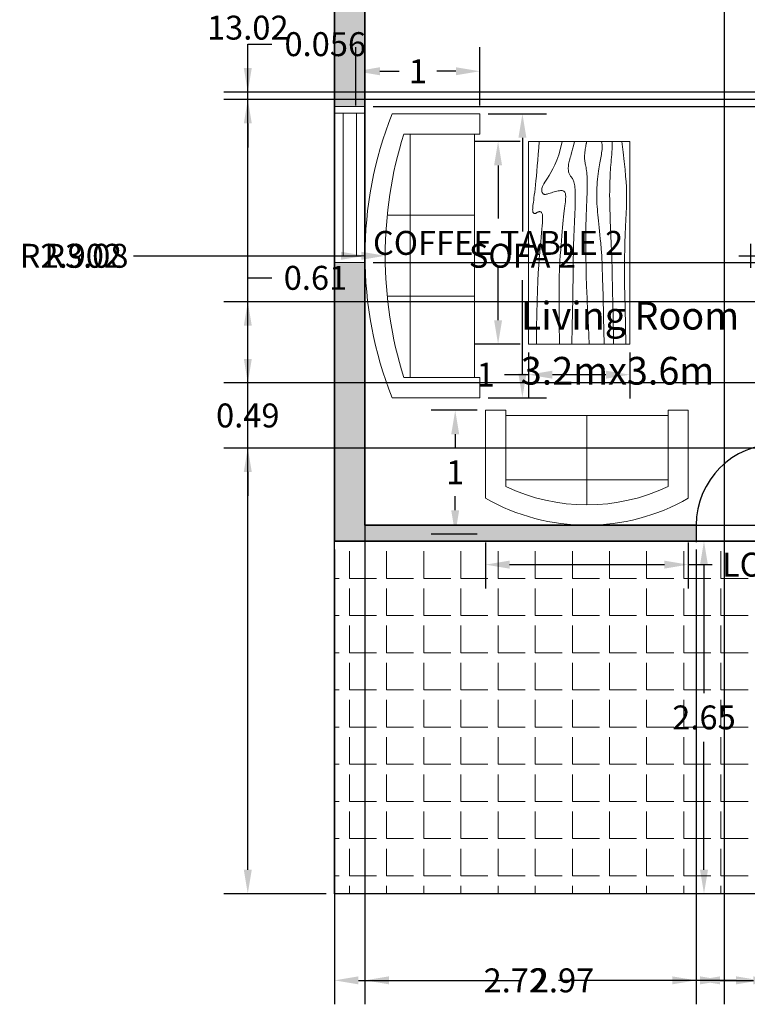
# Model space of a CAD drawing. Units: metres. Extents: x 35.2 to 46.4, y 446.1 to 460.8.
# Tile 1 of 6: x 35.2 to 40.7, y 446.1 to 453.5. Entities that reach past the tile are written whole.
import ezdxf

# ---------------------------------------------------------------- set-up
doc = ezdxf.new("R2010")
doc.units = ezdxf.units.M
for name, color, linetype, lineweight in [('A-ANNO-DIMS', 2, 'Continuous', 18), ('A-AREA-IDEN', 7, 'Continuous', 18), ('A-DOOR', 3, 'Continuous', 25), ('A-FLOR', 7, 'Continuous', 25), ('A-FLOR-PATT', 9, 'Continuous', 13), ('A-GLAZ', 4, 'Continuous', 18), ('A-WALL', 7, 'Continuous', 35), ('A-WALL-PATT', 252, 'Continuous', 13), ('FURNITURE', 53, 'Continuous', 18)]:
    doc.layers.add(name, color=color, linetype=linetype, lineweight=lineweight)
doc.styles.get("Standard").update_dxf_attribs({"font": 'calibri.ttf'})
doc.dimstyles.get("Standard").update_dxf_attribs({"dimtxt": 0.18, "dimasz": 0.18, "dimexe": 0.18, "dimexo": 0.0625, "dimgap": 0.09, "dimtad": 0, "dimtih": 1, "dimtoh": 1, "dimdec": 4, "dimzin": 0, "dimdsep": 46, "dimtxsty": 'Standard', "dimcen": 0.09, "dimadec": 0, "dimazin": 0, "dimtfac": 1, "dimtdec": 4, "dimtofl": 0, "dimtmove": 0, "dimatfit": 3, "dimfxl": 1, "dimtolj": 1, "dimtzin": 0, "dimarcsym": 0})

# ---------------------------------------------------------------- blocks, each defined once
blk = doc.blocks.new('*U4')
for p, q in [((-24, 0), (-24, -5)), ((0, 0), (0, -5))]:
    blk.add_line(p, q)
blk.add_lwpolyline([(0, 0), (0, 24), (-1.75, 24), (-1.75, 0)], close=True)
blk.add_arc((0, 0), 24, 90, 180)
blk = doc.blocks.new('Table - Rectangular Woodgrain 60 x 30 in.')
for p, q in [((0, 0), (0, -30)), ((60, 0), (0, 0)), ((60, -30), (60, 0)), ((0, -30), (60, -30))]:
    blk.add_line(p, q)
for points in [[(0, -2.4), (4.8155, -2.418), (9.0302, -2.4688), (12.709, -2.5477), (15.9167, -2.65), (18.7181, -2.7711), (21.1781, -2.9063), (23.3616, -3.0508), (25.3333, -3.2), (27.1477, -3.3495), (28.8172, -3.4958), (30.3437, -3.636), (31.7291, -3.7667), (32.9756, -3.8849), (34.0849, -3.9875), (35.059, -4.0714), (35.9, -4.1334), (36.6114, -4.1711), (37.2041, -4.1854), (37.6906, -4.1779), (38.0833, -4.15), (38.3948, -4.1034), (38.6375, -4.0396), (38.8239, -3.9602), (38.9666, -3.8667), (39.0764, -3.7608), (39.1573, -3.6448), (39.2116, -3.521), (39.2416, -3.3917), (39.2498, -3.2593), (39.2385, -3.1261), (39.21, -2.9944), (39.1666, -2.8667), (39.111, -2.7447), (39.0468, -2.6281), (38.978, -2.5163), (38.9083, -2.4083), (38.8418, -2.3035), (38.7823, -2.201), (38.7337, -2.1001), (38.7, -2), (38.6844, -1.9003), (38.6875, -1.8021), (38.7094, -1.707), (38.75, -1.6167), (38.8094, -1.5326), (38.8875, -1.4563), (38.9844, -1.3893), (39.1, -1.3333), (39.2351, -1.2896), (39.3937, -1.2583), (39.5804, -1.2396), (39.8, -1.2333), (40.057, -1.2396), (40.3562, -1.2583), (40.7023, -1.2896), (41.1, -1.3333), (41.5547, -1.3895), (42.0755, -1.4573), (42.6721, -1.5361), (43.3542, -1.625), (44.1316, -1.7233), (45.014, -1.8302), (46.0114, -1.9449), (47.1333, -2.0667), (48.3862, -2.1947), (49.7625, -2.3281), (51.2513, -2.4663), (52.8416, -2.6083), (54.5226, -2.7535), (56.2833, -2.9011), (58.1127, -3.0501), (60, -3.2)], [(0, -9.2), (6.5759, -9.0858), (11.9385, -9.0365), (16.2527, -9.0418), (19.6833, -9.0917), (22.3952, -9.1759), (24.5531, -9.2844), (26.322, -9.4069), (27.8666, -9.5333), (29.3241, -9.6553), (30.7203, -9.7719), (32.0532, -9.8837), (33.3208, -9.9917), (34.5213, -10.0965), (35.6526, -10.199), (36.7128, -10.2999), (37.7, -10.4), (38.6129, -10.4996), (39.4531, -10.5969), (40.223, -10.6895), (40.925, -10.775), (41.5613, -10.8512), (42.1344, -10.9156), (42.6465, -10.966), (43.1, -11), (43.4976, -11.0158), (43.8437, -11.0136), (44.143, -10.9942), (44.4, -10.9583), (44.6195, -10.9069), (44.8062, -10.8406), (44.9648, -10.7603), (45.1, -10.6667), (45.2155, -10.5598), (45.3114, -10.4365), (45.3871, -10.2929), (45.4416, -10.125), (45.4743, -9.929), (45.4844, -9.7011), (45.4709, -9.4371), (45.4333, -9.1333), (45.3716, -8.7883), (45.2896, -8.4104), (45.1919, -8.0107), (45.0833, -7.6), (44.9685, -7.1893), (44.8521, -6.7896), (44.7388, -6.4117), (44.6333, -6.0667), (44.54, -5.7628), (44.4614, -5.4979), (44.4001, -5.2675), (44.3583, -5.0667), (44.3384, -4.8909), (44.3427, -4.7354), (44.3736, -4.5956), (44.4333, -4.4667), (44.5236, -4.3453), (44.6427, -4.2333), (44.7884, -4.1339), (44.9583, -4.05), (45.1501, -3.9849), (45.3614, -3.9417), (45.59, -3.9234), (45.8333, -3.9333), (46.0915, -3.9749), (46.3734, -4.0531), (46.6906, -4.1736), (47.0542, -4.3417), (47.4756, -4.5629), (47.9661, -4.8427), (48.5372, -5.1866), (49.2, -5.6), (49.9676, -6.0844), (50.8594, -6.625), (51.8965, -7.2031), (53.1, -7.8), (54.491, -8.3969), (56.0906, -8.975), (57.9199, -9.5156), (60, -10)], [(0, -12.8), (5.1847, -12.9322), (9.6213, -13.0323), (13.3963, -13.1059), (16.5958, -13.1583), (19.3063, -13.1952), (21.614, -13.2219), (23.6054, -13.2439), (25.3666, -13.2667), (26.9728, -13.2947), (28.4531, -13.3281), (29.8256, -13.3663), (31.1083, -13.4083), (32.3191, -13.4535), (33.476, -13.501), (34.597, -13.5501), (35.7, -13.6), (36.7984, -13.6497), (37.8875, -13.6979), (38.9578, -13.743), (40, -13.7833), (41.0047, -13.8174), (41.9625, -13.8438), (42.864, -13.8607), (43.7, -13.8667), (44.4631, -13.8604), (45.1552, -13.8417), (45.7801, -13.8104), (46.3416, -13.7667), (46.8439, -13.7104), (47.2906, -13.6417), (47.6858, -13.5604), (48.0333, -13.4667), (48.3375, -13.3608), (48.6042, -13.2448), (48.8396, -13.121), (49.05, -12.9917), (49.2417, -12.8593), (49.4208, -12.7261), (49.5937, -12.5944), (49.7667, -12.4667), (49.9452, -12.3451), (50.1323, -12.2313), (50.3303, -12.1268), (50.5416, -12.0333), (50.7686, -11.9524), (51.0135, -11.8854), (51.2788, -11.8341), (51.5666, -11.8), (51.8785, -11.7843), (52.2116, -11.7865), (52.562, -11.8059), (52.926, -11.8417), (53.2998, -11.8931), (53.6795, -11.9594), (54.0614, -12.0397), (54.4416, -12.1333), (54.8223, -12.2401), (55.2293, -12.3625), (55.6942, -12.5037), (56.2489, -12.6667), (56.9251, -12.8547), (57.7545, -13.0708), (58.7689, -13.3182), (60, -13.6)], [(0, -18), (5.124, -17.7273), (9.6609, -17.5057), (13.6705, -17.3303), (17.2125, -17.1958), (20.3467, -17.0973), (23.1328, -17.0297), (25.6307, -16.9878), (27.9, -16.9667), (29.9928, -16.9617), (31.9302, -16.9703), (33.7254, -16.9907), (35.3917, -17.0208), (36.9423, -17.0588), (38.3906, -17.1026), (39.7499, -17.1503), (41.0333, -17.2), (42.2519, -17.2496), (43.4073, -17.2969), (44.4986, -17.3395), (45.525, -17.375), (46.4858, -17.4012), (47.3802, -17.4156), (48.2074, -17.416), (48.9667, -17.4), (49.6583, -17.3662), (50.2872, -17.3167), (50.8595, -17.2547), (51.3812, -17.1833), (51.8584, -17.1057), (52.2971, -17.025), (52.7034, -16.9443), (53.0833, -16.8667), (53.443, -16.7951), (53.789, -16.7313), (54.128, -16.6768), (54.4666, -16.6334), (54.8115, -16.6024), (55.1693, -16.5854), (55.5465, -16.5841), (55.95, -16.6), (56.3828, -16.6337), (56.8346, -16.6823), (57.2915, -16.7418), (57.7396, -16.8084), (58.165, -16.878), (58.5539, -16.9469), (58.8924, -17.0111), (59.1666, -17.0667), (59.3679, -17.1107), (59.5078, -17.1438), (59.6032, -17.1675), (59.6708, -17.1833), (59.7275, -17.193), (59.7901, -17.1979), (59.8753, -17.1998), (60, -17.2)], [(0, -22.4), (8.0098, -22.2501), (14.4094, -22.1011), (19.4168, -21.9535), (23.25, -21.8083), (26.1269, -21.6663), (28.2656, -21.5281), (29.884, -21.3947), (31.2, -21.2667), (32.3967, -21.1448), (33.5172, -21.0292), (34.5697, -20.9198), (35.5625, -20.8167), (36.5037, -20.7198), (37.4015, -20.6292), (38.2642, -20.5448), (39.1, -20.4667), (39.9164, -20.3951), (40.7187, -20.3313), (41.5117, -20.2768), (42.3, -20.2333), (43.0883, -20.2024), (43.8812, -20.1854), (44.6836, -20.1841), (45.5, -20.2), (46.3328, -20.234), (47.1747, -20.2844), (48.0163, -20.3488), (48.8479, -20.425), (49.66, -20.5106), (50.4429, -20.6031), (51.1872, -20.7004), (51.8833, -20.8), (52.5246, -20.8999), (53.1166, -20.9995), (53.6681, -21.0983), (54.1875, -21.1958), (54.6834, -21.2919), (55.1646, -21.3859), (55.6394, -21.4777), (56.1167, -21.5667), (56.6028, -21.6515), (57.0961, -21.7266), (57.5929, -21.7852), (58.0896, -21.8208), (58.5823, -21.8268), (59.0674, -21.7964), (59.5412, -21.723), (60, -21.6)], [(0, -25.2), (8.6355, -25.0504), (15.7026, -24.9031), (21.4049, -24.7606), (25.9458, -24.625), (29.529, -24.4988), (32.3578, -24.3844), (34.6359, -24.284), (36.5667, -24.2), (38.3213, -24.1341), (39.9417, -24.0854), (41.437, -24.0523), (42.8167, -24.0333), (44.0901, -24.0268), (45.2667, -24.0313), (46.3557, -24.0451), (47.3667, -24.0667), (48.309, -24.0947), (49.1928, -24.1287), (50.0284, -24.168), (50.826, -24.2125), (51.5959, -24.2617), (52.3483, -24.3151), (53.0935, -24.3725), (53.8417, -24.4334), (54.6009, -24.497), (55.3699, -24.561), (56.1454, -24.6226), (56.9239, -24.6792), (57.7021, -24.7279), (58.4764, -24.7662), (59.2435, -24.7911), (60, -24.8)], [(0, -28.8), (5.6867, -28.6681), (10.45, -28.5698), (14.407, -28.5012), (17.675, -28.4584), (20.3711, -28.4374), (22.6125, -28.4344), (24.5164, -28.4455), (26.2, -28.4667), (27.762, -28.4947), (29.2276, -28.5281), (30.6033, -28.5663), (31.8958, -28.6084), (33.1118, -28.6535), (34.2578, -28.7011), (35.3405, -28.7501), (36.3666, -28.8), (37.3443, -28.8497), (38.288, -28.8974), (39.2137, -28.9412), (40.1375, -28.9792), (41.0753, -29.0093), (42.0432, -29.0297), (43.0572, -29.0384), (44.1333, -29.0333), (45.2936, -29.0114), (46.5843, -28.9641), (48.0579, -28.8816), (49.7666, -28.7542), (51.7629, -28.5721), (54.0989, -28.3255), (56.8272, -28.0048), (60, -27.6)]]:
    blk.add_lwpolyline(points)
blk = doc.blocks.new('Sofa - Roundback 7 ft.')
for p, q in [((-12.00002, -32.4421), (-12.00003, -6.5971)), ((11.99997, -32.4421), (11.99998, -6.5971)), ((-36.000027, -34), (-36.000027, -11.4696)), ((35.99998, -34), (35.99998, -11.4696)), ((-35.999844, -13.3819), (35.9998, -13.3819)), ((-36.000027, -32.4421), (35.99998, -32.4421))]:
    blk.add_line(p, q)
for points in [[(-36.000027, -34), (-42.000027, -34), (-42.000027, -8)], [(41.99998, -8), (41.99998, -34), (35.99998, -34)]]:
    blk.add_lwpolyline(points)
for centre, radius, start, end in [((0, -114.25), 114.25, 68.43141, 111.5686), ((-0.00001, -127.1968), 121.1968, 72.72033, 107.2797)]:
    blk.add_arc(centre, radius, start, end)
blk = doc.blocks.new('Sofa - Roundback Loveseat 5 ft.')
for p, q in [((0, -32.44198), (0, -5.99998)), ((-24, -33.99998), (-24, -11.46958)), ((24.00004, -33.99998), (24.00004, -11.46958)), ((-23.9998, -13.38178), (23.99986, -13.38178)), ((-24, -32.44198), (24.00004, -32.44198))]:
    blk.add_line(p, q)
for points in [[(-24, -33.99998), (-30, -33.99998), (-30, -7.99998)], [(30.00004, -7.99998), (30.00004, -33.99998), (24.00004, -33.99998)]]:
    blk.add_lwpolyline(points)
for centre, radius, start, end in [((0, -60.24998), 60.24998, 60.13715, 119.8628), ((0, -61.38438), 55.38444, 64.32083, 115.6792)]:
    blk.add_arc(centre, radius, start, end)
blk = doc.blocks.new('WIN-1172')
for p, q in [((0, 1.1716), (0.23, 1.1716)), ((0, 1.1716), (0, 0)), ((0, 1.1216), (0.23, 1.1216)), ((0.065, 1.1216), (0.065, 0.05)), ((0.165, 1.1216), (0.165, 0.05)), ((0.23, 1.1716), (0.23, 0)), ((0.23, 0.05), (0, 0.05)), ((0.23, 0), (0, 0))]:
    blk.add_line(p, q)
blk = doc.blocks.new('*D141')
at = {"layer": 'A-ANNO-DIMS', "color": 0, "lineweight": -2, "transparency": 16777216}
for p, q in [((39.0034, 452.5589), (38.6573, 452.5589)), ((38.8373, 452.3789), (38.8373, 451.9792)), ((38.8373, 451.2149), (38.8373, 451.6147)), ((39.0034, 451.0349), (38.6573, 451.0349))]:
    blk.add_line(p, q, dxfattribs=at)
at = {"layer": 'A-ANNO-DIMS', "color": 0, "transparency": 16777216}
for points in [[(38.8073, 452.3789), (38.8673, 452.3789), (38.8373, 452.5589)], [(38.8073, 451.2149), (38.8673, 451.2149), (38.8373, 451.0349)]]:
    blk.add_solid(points, dxfattribs=at)
at = {"layer": 'Defpoints', "color": 0, "transparency": 16777216}
for p in [(38.8373, 452.5589), (39.0659, 452.5589), (39.0659, 451.0349)]:
    blk.add_point(p, dxfattribs=at)
at = {"layer": 'A-ANNO-DIMS', "color": 0, "transparency": 16777216, "insert": (38.8373, 451.7969), "char_height": 0.18, "attachment_point": 5}
blk.add_mtext('\\A1;COFFEE TABLE 2', dxfattribs=at)
blk = doc.blocks.new('*D142')
at = {"layer": 'A-ANNO-DIMS', "color": 0, "lineweight": -2, "transparency": 16777216}
for p, q in [((39.0659, 450.9724), (39.0659, 450.6263)), ((39.8279, 450.9724), (39.8279, 450.6263)), ((39.0659, 450.8063), (38.8859, 450.8063)), ((39.6479, 450.8063), (39.2459, 450.8063))]:
    blk.add_line(p, q, dxfattribs=at)
at = {"layer": 'A-ANNO-DIMS', "color": 0, "transparency": 16777216}
for points in [[(39.2459, 450.8363), (39.2459, 450.7763), (39.0659, 450.8063)], [(39.6479, 450.8363), (39.6479, 450.7763), (39.8279, 450.8063)]]:
    blk.add_solid(points, dxfattribs=at)
at = {"layer": 'Defpoints', "color": 0, "transparency": 16777216}
for p in [(39.0659, 451.0349), (39.8279, 451.0349), (39.0659, 450.8063)]:
    blk.add_point(p, dxfattribs=at)
at = {"layer": 'A-ANNO-DIMS', "color": 0, "transparency": 16777216, "insert": (38.7437, 450.8063), "char_height": 0.18, "attachment_point": 5}
blk.add_mtext('\\A1;1', dxfattribs=at)
blk = doc.blocks.new('*D143')
at = {"layer": 'A-ANNO-DIMS', "color": 0, "lineweight": -2, "transparency": 16777216}
for p, q in [((38.7627, 452.7669), (39.2002, 452.7669)), ((39.0202, 452.5869), (39.0202, 451.8824)), ((39.0202, 450.8133), (39.0202, 451.5179)), ((38.7627, 450.6333), (39.2002, 450.6333))]:
    blk.add_line(p, q, dxfattribs=at)
at = {"layer": 'A-ANNO-DIMS', "color": 0, "transparency": 16777216}
for points in [[(38.9902, 452.5869), (39.0502, 452.5869), (39.0202, 452.7669)], [(38.9902, 450.8133), (39.0502, 450.8133), (39.0202, 450.6333)]]:
    blk.add_solid(points, dxfattribs=at)
at = {"layer": 'Defpoints', "color": 0, "transparency": 16777216}
for p in [(38.7002, 452.7669), (39.0202, 452.7669), (38.7002, 450.6333)]:
    blk.add_point(p, dxfattribs=at)
at = {"layer": 'A-ANNO-DIMS', "color": 0, "transparency": 16777216, "insert": (39.0202, 451.7001), "char_height": 0.18, "attachment_point": 5}
blk.add_mtext('\\A1;SOFA 2', dxfattribs=at)
blk = doc.blocks.new('*D144')
at = {"layer": 'A-ANNO-DIMS', "color": 0, "lineweight": -2, "transparency": 16777216}
for p, q in [((37.7689, 452.8294), (37.7689, 453.267)), ((38.7002, 452.8294), (38.7002, 453.267)), ((37.9489, 453.087), (38.0924, 453.087)), ((38.5202, 453.087), (38.3767, 453.087))]:
    blk.add_line(p, q, dxfattribs=at)
at = {"layer": 'A-ANNO-DIMS', "color": 0, "transparency": 16777216}
for points in [[(37.9489, 453.117), (37.9489, 453.057), (37.7689, 453.087)], [(38.5202, 453.117), (38.5202, 453.057), (38.7002, 453.087)]]:
    blk.add_solid(points, dxfattribs=at)
at = {"layer": 'Defpoints', "color": 0, "transparency": 16777216}
for p in [(37.7689, 453.087), (37.7689, 452.7669), (38.7002, 452.7669)]:
    blk.add_point(p, dxfattribs=at)
at = {"layer": 'A-ANNO-DIMS', "color": 0, "transparency": 16777216, "insert": (38.2345, 453.087), "char_height": 0.18, "attachment_point": 5}
blk.add_mtext('\\A1;1', dxfattribs=at)
blk = doc.blocks.new('*D147')
at = {"layer": 'A-ANNO-DIMS', "color": 0, "lineweight": -2, "transparency": 16777216}
for p, q in [((38.7435, 449.5445), (38.7435, 449.1984)), ((40.2675, 449.5445), (40.2675, 449.1984)), ((38.9235, 449.3784), (40.0875, 449.3784)), ((40.2675, 449.3784), (40.4475, 449.3784))]:
    blk.add_line(p, q, dxfattribs=at)
at = {"layer": 'A-ANNO-DIMS', "color": 0, "transparency": 16777216}
for points in [[(38.9235, 449.4084), (38.9235, 449.3484), (38.7435, 449.3784)], [(40.0875, 449.4084), (40.0875, 449.3484), (40.2675, 449.3784)]]:
    blk.add_solid(points, dxfattribs=at)
at = {"layer": 'Defpoints', "color": 0, "transparency": 16777216}
for p in [(38.7435, 449.607), (40.2675, 449.607), (40.2675, 449.3784)]:
    blk.add_point(p, dxfattribs=at)
at = {"layer": 'A-ANNO-DIMS', "color": 0, "transparency": 16777216, "insert": (41.2103, 449.3784), "char_height": 0.18, "attachment_point": 5}
blk.add_mtext('\\A1;LOVESEAT 2', dxfattribs=at)
blk = doc.blocks.new('*D148')
at = {"layer": 'A-ANNO-DIMS', "color": 0, "lineweight": -2, "transparency": 16777216}
for p, q in [((38.681, 450.5384), (38.3349, 450.5384)), ((38.5149, 450.3584), (38.5149, 450.2529)), ((38.5149, 449.787), (38.5149, 449.8925)), ((38.681, 449.607), (38.3349, 449.607))]:
    blk.add_line(p, q, dxfattribs=at)
at = {"layer": 'A-ANNO-DIMS', "color": 0, "transparency": 16777216}
for points in [[(38.4849, 450.3584), (38.5449, 450.3584), (38.5149, 450.5384)], [(38.4849, 449.787), (38.5449, 449.787), (38.5149, 449.607)]]:
    blk.add_solid(points, dxfattribs=at)
at = {"layer": 'Defpoints', "color": 0, "transparency": 16777216}
for p in [(38.7435, 450.5384), (38.5149, 449.607), (38.7435, 449.607)]:
    blk.add_point(p, dxfattribs=at)
at = {"layer": 'A-ANNO-DIMS', "color": 0, "transparency": 16777216, "insert": (38.5149, 450.0727), "char_height": 0.18, "attachment_point": 5}
blk.add_mtext('\\A1;1', dxfattribs=at)
blk = doc.blocks.new('*D152')
at = {"layer": 'A-ANNO-DIMS', "color": 0, "lineweight": -2, "transparency": 16777216}
for p, q in [((37.5441, 459.9248), (36.7754, 459.9248)), ((36.9554, 459.7448), (36.9554, 453.597)), ((36.9554, 447.0848), (36.9554, 453.2326)), ((37.5441, 446.9048), (36.7754, 446.9048))]:
    blk.add_line(p, q, dxfattribs=at)
at = {"layer": 'A-ANNO-DIMS', "color": 0, "transparency": 16777216}
for points in [[(36.9254, 459.7448), (36.9854, 459.7448), (36.9554, 459.9248)], [(36.9254, 447.0848), (36.9854, 447.0848), (36.9554, 446.9048)]]:
    blk.add_solid(points, dxfattribs=at)
at = {"layer": 'Defpoints', "color": 0, "transparency": 16777216}
for p in [(36.9554, 459.9248), (37.6066, 459.9248), (37.6066, 446.9048)]:
    blk.add_point(p, dxfattribs=at)
at = {"layer": 'A-ANNO-DIMS', "color": 0, "transparency": 16777216, "insert": (36.9554, 453.4148), "char_height": 0.18, "attachment_point": 5}
blk.add_mtext('\\A1;13.02', dxfattribs=at)
blk = doc.blocks.new('*D154')
at = {"layer": 'A-ANNO-DIMS', "color": 0, "lineweight": -2, "transparency": 16777216}
for p, q in [((40.9741, 449.5548), (40.2054, 449.5548)), ((40.3854, 449.3748), (40.3854, 448.412)), ((40.3854, 447.0848), (40.3854, 448.0476)), ((40.9741, 446.9048), (40.2054, 446.9048))]:
    blk.add_line(p, q, dxfattribs=at)
at = {"layer": 'A-ANNO-DIMS', "color": 0, "transparency": 16777216}
for points in [[(40.3554, 449.3748), (40.4154, 449.3748), (40.3854, 449.5548)], [(40.3554, 447.0848), (40.4154, 447.0848), (40.3854, 446.9048)]]:
    blk.add_solid(points, dxfattribs=at)
at = {"layer": 'Defpoints', "color": 0, "transparency": 16777216}
for p in [(40.3854, 449.5548), (41.0366, 449.5548), (41.0366, 446.9048)]:
    blk.add_point(p, dxfattribs=at)
at = {"layer": 'A-ANNO-DIMS', "color": 0, "transparency": 16777216, "insert": (40.3854, 448.2298), "char_height": 0.18, "attachment_point": 5}
blk.add_mtext('\\A1;2.65', dxfattribs=at)
blk = doc.blocks.new('*D155')
at = {"layer": 'A-ANNO-DIMS', "color": 0, "lineweight": -2, "transparency": 16777216}
for p, q in [((37.8991, 451.6506), (45.8178, 451.6506)), ((45.6378, 451.4706), (45.6378, 450.8449)), ((45.6378, 449.8548), (45.6378, 450.4805)), ((37.8991, 449.6748), (45.8178, 449.6748))]:
    blk.add_line(p, q, dxfattribs=at)
at = {"layer": 'A-ANNO-DIMS', "color": 0, "transparency": 16777216}
for points in [[(45.6078, 451.4706), (45.6678, 451.4706), (45.6378, 451.6506)], [(45.6078, 449.8548), (45.6678, 449.8548), (45.6378, 449.6748)]]:
    blk.add_solid(points, dxfattribs=at)
at = {"layer": 'Defpoints', "color": 0, "transparency": 16777216}
for p in [(37.8366, 451.6506), (45.6378, 451.6506), (37.8366, 449.6748)]:
    blk.add_point(p, dxfattribs=at)
at = {"layer": 'A-ANNO-DIMS', "color": 0, "transparency": 16777216, "insert": (45.6378, 450.6627), "char_height": 0.18, "attachment_point": 5}
blk.add_mtext('\\A1;1.976', dxfattribs=at)
blk = doc.blocks.new('*D156')
at = {"layer": 'A-ANNO-DIMS', "color": 0, "lineweight": -2, "transparency": 16777216}
for p, q in [((37.8991, 455.122), (45.8178, 455.122)), ((45.6378, 454.942), (45.6378, 454.1543)), ((45.6378, 453.0022), (45.6378, 453.7898)), ((37.8991, 452.8222), (45.8178, 452.8222))]:
    blk.add_line(p, q, dxfattribs=at)
at = {"layer": 'A-ANNO-DIMS', "color": 0, "transparency": 16777216}
for points in [[(45.6078, 454.942), (45.6678, 454.942), (45.6378, 455.122)], [(45.6078, 453.0022), (45.6678, 453.0022), (45.6378, 452.8222)]]:
    blk.add_solid(points, dxfattribs=at)
at = {"layer": 'Defpoints', "color": 0, "transparency": 16777216}
for p in [(37.8366, 455.122), (45.6378, 455.122), (37.8366, 452.8222)]:
    blk.add_point(p, dxfattribs=at)
at = {"layer": 'A-ANNO-DIMS', "color": 0, "transparency": 16777216, "insert": (45.6378, 453.9721), "char_height": 0.18, "attachment_point": 5}
blk.add_mtext('\\A1;2.3', dxfattribs=at)
blk = doc.blocks.new('*D167')
at = {"layer": 'A-ANNO-DIMS', "color": 0, "lineweight": -2, "transparency": 16777216}
for p, q in [((37.8366, 459.6323), (37.8366, 446.0736)), ((40.8069, 459.6323), (40.8069, 446.0736)), ((38.0166, 446.2536), (38.9948, 446.2536)), ((40.6269, 446.2536), (39.6486, 446.2536))]:
    blk.add_line(p, q, dxfattribs=at)
at = {"layer": 'A-ANNO-DIMS', "color": 0, "transparency": 16777216}
for points in [[(38.0166, 446.2836), (38.0166, 446.2236), (37.8366, 446.2536)], [(40.6269, 446.2836), (40.6269, 446.2236), (40.8069, 446.2536)]]:
    blk.add_solid(points, dxfattribs=at)
at = {"layer": 'Defpoints', "color": 0, "transparency": 16777216}
for p in [(37.8366, 459.6948), (40.8069, 459.6948), (40.8069, 446.2536)]:
    blk.add_point(p, dxfattribs=at)
at = {"layer": 'A-ANNO-DIMS', "color": 0, "transparency": 16777216, "insert": (39.3217, 446.2536), "char_height": 0.18, "attachment_point": 5}
blk.add_mtext('\\A1;2.97', dxfattribs=at)
blk = doc.blocks.new('*D169')
at = {"layer": 'A-ANNO-DIMS', "color": 0, "lineweight": -2, "transparency": 16777216}
for p, q in [((40.536595, 457.132279), (40.536595, 446.073579)), ((41.656595, 457.132279), (41.656595, 446.073579)), ((40.356595, 446.253579), (40.176595, 446.253579)), ((41.836595, 446.253579), (42.016595, 446.253579))]:
    blk.add_line(p, q, dxfattribs=at)
at = {"layer": 'A-ANNO-DIMS', "color": 0, "transparency": 16777216}
for points in [[(40.356595, 446.283579), (40.356595, 446.223579), (40.536595, 446.253579)], [(41.836595, 446.283579), (41.836595, 446.223579), (41.656595, 446.253579)]]:
    blk.add_solid(points, dxfattribs=at)
at = {"layer": 'Defpoints', "color": 0, "transparency": 16777216}
for p in [(40.536595, 457.194779), (41.656595, 457.194779), (41.656595, 446.253579)]:
    blk.add_point(p, dxfattribs=at)
at = {"layer": 'A-ANNO-DIMS', "color": 0, "transparency": 16777216, "insert": (41.096595, 446.253579), "char_height": 0.18, "attachment_point": 5}
blk.add_mtext('\\A1;1.12', dxfattribs=at)
blk = doc.blocks.new('*D173')
at = {"layer": 'A-ANNO-DIMS', "color": 0, "lineweight": -2, "transparency": 16777216}
for p, q in [((37.6066, 449.4923), (37.6066, 446.0736)), ((40.327, 449.4923), (40.327, 446.0736)), ((37.7866, 446.2536), (38.6412, 446.2536)), ((40.147, 446.2536), (39.2924, 446.2536))]:
    blk.add_line(p, q, dxfattribs=at)
at = {"layer": 'A-ANNO-DIMS', "color": 0, "transparency": 16777216}
for points in [[(37.7866, 446.2836), (37.7866, 446.2236), (37.6066, 446.2536)], [(40.147, 446.2836), (40.147, 446.2236), (40.327, 446.2536)]]:
    blk.add_solid(points, dxfattribs=at)
at = {"layer": 'Defpoints', "color": 0, "transparency": 16777216}
for p in [(37.6066, 449.5548), (40.327, 449.5548), (40.327, 446.2536)]:
    blk.add_point(p, dxfattribs=at)
at = {"layer": 'A-ANNO-DIMS', "color": 0, "transparency": 16777216, "insert": (38.9668, 446.2536), "char_height": 0.18, "attachment_point": 5}
blk.add_mtext('\\A1;2.72', dxfattribs=at)
blk = doc.blocks.new('*D174')
at = {"layer": 'A-ANNO-DIMS', "color": 0, "lineweight": -2, "transparency": 16777216}
for p, q in [((40.327, 449.4923), (40.327, 446.0736)), ((40.9366, 449.4923), (40.9366, 446.0736)), ((40.507, 446.2536), (40.7566, 446.2536)), ((40.9366, 446.2536), (41.1166, 446.2536))]:
    blk.add_line(p, q, dxfattribs=at)
at = {"layer": 'A-ANNO-DIMS', "color": 0, "transparency": 16777216}
for points in [[(40.507, 446.2836), (40.507, 446.2236), (40.327, 446.2536)], [(40.7566, 446.2836), (40.7566, 446.2236), (40.9366, 446.2536)]]:
    blk.add_solid(points, dxfattribs=at)
at = {"layer": 'Defpoints', "color": 0, "transparency": 16777216}
for p in [(40.327, 449.5548), (40.9366, 449.5548), (40.9366, 446.2536)]:
    blk.add_point(p, dxfattribs=at)
at = {"layer": 'A-ANNO-DIMS', "color": 0, "transparency": 16777216, "insert": (41.4453, 446.2536), "char_height": 0.18, "attachment_point": 5}
blk.add_mtext('\\A1;0.61', dxfattribs=at)
blk = doc.blocks.new('*D180')
at = {"layer": 'A-ANNO-DIMS', "color": 0, "lineweight": -2, "transparency": 16777216}
for p, q in [((36.9554, 450.9246), (36.9554, 451.1046)), ((42.0566, 450.7446), (36.7754, 450.7446)), ((42.0566, 450.2548), (36.7754, 450.2548)), ((36.9554, 450.0748), (36.9554, 449.8948))]:
    blk.add_line(p, q, dxfattribs=at)
at = {"layer": 'A-ANNO-DIMS', "color": 0, "transparency": 16777216}
for points in [[(36.9254, 450.9246), (36.9854, 450.9246), (36.9554, 450.7446)], [(36.9254, 450.0748), (36.9854, 450.0748), (36.9554, 450.2548)]]:
    blk.add_solid(points, dxfattribs=at)
at = {"layer": 'Defpoints', "color": 0, "transparency": 16777216}
for p in [(36.9554, 450.7446), (42.1191, 450.7446), (42.1191, 450.2548)]:
    blk.add_point(p, dxfattribs=at)
at = {"layer": 'A-ANNO-DIMS', "color": 0, "transparency": 16777216, "insert": (36.9554, 450.4997), "char_height": 0.18, "attachment_point": 5}
blk.add_mtext('\\A1;0.49', dxfattribs=at)
blk = doc.blocks.new('*D181')
at = {"layer": 'A-ANNO-DIMS', "color": 0, "lineweight": -2, "transparency": 16777216}
for p, q in [((36.9554, 451.3542), (36.9554, 451.5342)), ((36.9554, 451.5342), (37.1354, 451.5342)), ((42.0566, 451.3542), (36.7754, 451.3542)), ((36.9554, 450.9246), (36.9554, 451.1742)), ((42.0566, 450.7446), (36.7754, 450.7446))]:
    blk.add_line(p, q, dxfattribs=at)
at = {"layer": 'A-ANNO-DIMS', "color": 0, "transparency": 16777216}
for points in [[(36.9254, 451.1742), (36.9854, 451.1742), (36.9554, 451.3542)], [(36.9254, 450.9246), (36.9854, 450.9246), (36.9554, 450.7446)]]:
    blk.add_solid(points, dxfattribs=at)
at = {"layer": 'Defpoints', "color": 0, "transparency": 16777216}
for p in [(36.9554, 451.3542), (42.1191, 451.3542), (42.1191, 450.7446)]:
    blk.add_point(p, dxfattribs=at)
at = {"layer": 'A-ANNO-DIMS', "color": 0, "transparency": 16777216, "insert": (37.4641, 451.5342), "char_height": 0.18, "attachment_point": 5}
blk.add_mtext('\\A1;0.61', dxfattribs=at)
blk = doc.blocks.new('*D186')
at = {"layer": 'A-ANNO-DIMS', "color": 0, "lineweight": -2, "transparency": 16777216}
for p, q in [((36.9554, 453.1107), (36.9554, 453.2907)), ((36.9554, 453.2907), (37.1354, 453.2907)), ((42.0566, 452.9307), (36.7754, 452.9307)), ((42.0566, 452.8748), (36.7754, 452.8748)), ((36.9554, 452.6948), (36.9554, 452.5148))]:
    blk.add_line(p, q, dxfattribs=at)
at = {"layer": 'A-ANNO-DIMS', "color": 0, "transparency": 16777216}
for points in [[(36.9254, 453.1107), (36.9854, 453.1107), (36.9554, 452.9307)], [(36.9254, 452.6948), (36.9854, 452.6948), (36.9554, 452.8748)]]:
    blk.add_solid(points, dxfattribs=at)
at = {"layer": 'Defpoints', "color": 0, "transparency": 16777216}
for p in [(36.9554, 452.9307), (42.1191, 452.9307), (42.1191, 452.8748)]:
    blk.add_point(p, dxfattribs=at)
at = {"layer": 'A-ANNO-DIMS', "color": 0, "transparency": 16777216, "insert": (37.538, 453.2907), "char_height": 0.18, "attachment_point": 5}
blk.add_mtext('\\A1;0.056', dxfattribs=at)
blk = doc.blocks.new('*D187')
at = {"layer": 'A-ANNO-DIMS', "color": 0, "lineweight": -2, "transparency": 16777216}
for p, q in [((41.0674, 451.6101), (41.0674, 451.7901)), ((36.142, 451.6999), (37.809, 451.7)), ((40.9774, 451.7001), (41.1574, 451.7001))]:
    blk.add_line(p, q, dxfattribs=at)
at = {"layer": 'A-ANNO-DIMS', "color": 0, "transparency": 16777216}
blk.add_solid([(37.809, 451.73), (37.809, 451.67), (37.989, 451.7)], dxfattribs=at)
at = {"layer": 'Defpoints', "color": 0, "transparency": 16777216}
for p in [(37.989, 451.7), (41.0674, 451.7001)]:
    blk.add_point(p, dxfattribs=at)
at = {"layer": 'A-ANNO-DIMS', "color": 0, "transparency": 16777216, "insert": (35.7413, 451.6999), "char_height": 0.18, "attachment_point": 5}
blk.add_mtext('\\A1;R3.08', dxfattribs=at)
blk = doc.blocks.new('*D188')
at = {"layer": 'A-ANNO-DIMS', "color": 0, "lineweight": -2, "transparency": 16777216}
for p, q in [((40.7385, 451.6101), (40.7385, 451.7901)), ((36.0954, 451.6999), (37.6566, 451.7)), ((40.6485, 451.7001), (40.8285, 451.7001))]:
    blk.add_line(p, q, dxfattribs=at)
at = {"layer": 'A-ANNO-DIMS', "color": 0, "transparency": 16777216}
blk.add_solid([(37.6566, 451.73), (37.6566, 451.67), (37.8366, 451.7)], dxfattribs=at)
at = {"layer": 'Defpoints', "color": 0, "transparency": 16777216}
for p in [(37.8366, 451.7), (40.7385, 451.7001)]:
    blk.add_point(p, dxfattribs=at)
at = {"layer": 'A-ANNO-DIMS', "color": 0, "transparency": 16777216, "insert": (35.625, 451.6999), "char_height": 0.18, "attachment_point": 5}
blk.add_mtext('\\A1;R2.902', dxfattribs=at)

msp = doc.modelspace()

# ---------------------------------------------------------------- hatches: boundary and pattern name
at = {"layer": 'A-FLOR-PATT'}
h = msp.add_hatch(dxfattribs=at)
h.set_pattern_fill('ANGLE', color=256, scale=0.04)
h.set_pattern_definition([(0, (0, 0), (0, 0.2794), [0.2032, -0.0762]), (90, (0, 0), (-0.2794, 0), [0.2032, -0.0762])])
h.paths.add_polyline_path([(41.0366, 449.5548), (37.6066, 449.5548), (37.6066, 446.9048), (41.0366, 446.9048)])
at = {"layer": 'A-WALL-PATT'}
h = msp.add_hatch(color=256, dxfattribs=at)
h.dxf.hatch_style = 1
h.paths.add_polyline_path([(37.8366, 451.6506), (37.6066, 451.6506), (37.6066, 449.5548), (40.327, 449.5548), (40.327, 449.6748), (37.8366, 449.6748)])
h.paths.add_polyline_path([(37.8366, 455.122), (37.6066, 455.122), (37.6066, 452.8222), (37.8366, 452.8222)])
h.paths.add_polyline_path([(37.8366, 457.0257), (37.8366, 457.0747), (37.8341, 457.0771), (37.8366, 457.0796), (37.8366, 457.1285), (37.8341, 457.131), (37.8366, 457.1335), (37.8366, 457.1824), (37.8341, 457.1849), (37.8366, 457.1874), (37.8366, 457.2363), (37.8341, 457.2388), (37.8366, 457.2412), (37.8366, 457.2902), (37.8341, 457.2927), (37.8366, 457.2951), (37.8366, 457.3441), (37.8341, 457.3465), (37.8366, 457.349), (37.8366, 457.398), (37.8341, 457.4004), (37.8366, 457.4029), (37.8366, 457.4518), (37.8341, 457.4543), (37.8366, 457.4568), (37.8366, 457.5057), (37.8341, 457.5082), (37.8366, 457.5107), (37.8366, 457.5596), (37.8341, 457.5621), (37.8366, 457.5645), (37.8366, 457.6135), (37.8341, 457.6159), (37.8366, 457.6184), (37.8366, 457.6674), (37.8341, 457.6698), (37.8366, 457.6723), (37.8366, 457.7212), (37.8341, 457.7237), (37.8366, 457.7262), (37.8366, 457.7751), (37.8341, 457.7776), (37.8366, 457.7801), (37.8366, 457.829), (37.8341, 457.8315), (37.8366, 457.8339), (37.8366, 457.8829), (37.8341, 457.8854), (37.8366, 457.8878), (37.8366, 457.9368), (37.8341, 457.9392), (37.8366, 457.9417), (37.8366, 457.9906), (37.8341, 457.9931), (37.8366, 457.9956), (37.8366, 458.0445), (37.8341, 458.047), (37.8366, 458.0495), (37.8366, 458.0984), (37.8341, 458.1009), (37.8366, 458.1033), (37.8366, 458.1523), (37.8272, 458.1617), (37.6066, 458.1617), (37.6066, 456.2935), (37.8366, 456.2935), (37.8366, 457.0208), (37.8341, 457.0232)], flags=17)
h.paths.add_polyline_path([(40.8069, 459.9248), (37.6066, 459.9248), (37.6066, 459.3333), (37.8273, 459.3333), (37.8366, 459.3426), (37.8366, 459.3916), (37.8341, 459.394), (37.8366, 459.3965), (37.8366, 459.4455), (37.8341, 459.4479), (37.8366, 459.4504), (37.8366, 459.4993), (37.8341, 459.5018), (37.8366, 459.5043), (37.8366, 459.5532), (37.8341, 459.5557), (37.8366, 459.5582), (37.8366, 459.6071), (37.8341, 459.6096), (37.8366, 459.612), (37.8366, 459.661), (37.8341, 459.6634), (37.8366, 459.6659), (37.8366, 459.6948), (40.4166, 459.6948), (40.4166, 457.0748), (41.0366, 457.0748), (41.0366, 455.1347), (41.1566, 455.1347), (41.1566, 455.9748), (41.2566, 455.9748), (41.2566, 456.0948), (41.1566, 456.0948), (41.1566, 457.0748), (41.7766, 457.0748), (41.7766, 459.6948), (44.7566, 459.6948), (44.7566, 458.3327), (44.9866, 458.3327), (44.9866, 459.9248), (41.3784, 459.9248), (41.3784, 459.6948), (41.6566, 459.6948), (41.6566, 457.1948), (40.5366, 457.1948), (40.5366, 459.6948), (40.8069, 459.6948)])
h.paths.add_polyline_path([(42.1191, 452.2548), (41.9991, 452.2548), (41.9991, 451.3542), (42.1191, 451.3542)])

# ---------------------------------------------------------------- linework, layer by layer
at = {"layer": 'A-FLOR'}
msp.add_lwpolyline([(37.6066, 449.5548), (41.0366, 449.5548), (41.0366, 446.9048), (37.6066, 446.9048)], close=True, dxfattribs=at)
at = {"layer": 'A-WALL'}
for p, q in [((37.6066, 459.9248), (37.6066, 449.5548)), ((37.8366, 459.6948), (37.8366, 449.6748)), ((37.8366, 449.6748), (40.327, 449.6748)), ((37.6066, 449.5548), (40.327, 449.5548))]:
    msp.add_line(p, q, dxfattribs=at)

# ---------------------------------------------------------------- block references
at = {"layer": 'A-DOOR', "xscale": 0.0254, "yscale": 0.0254, "zscale": 0.0254}
msp.add_blockref('*U4', (40.9366, 449.6748), dxfattribs=at)
at = {"layer": 'A-GLAZ'}
msp.add_blockref('WIN-1172', (37.6066, 451.6506), dxfattribs=at)
at = {"layer": 'FURNITURE', "transparency": 33554521, "yscale": 0.0254, "zscale": 0.0254}
for name, p, xscale, rotation in [('Sofa - Roundback 7 ft.', (37.8366, 451.7001), 0.0254, 90), ('Table - Rectangular Woodgrain 60 x 30 in.', (39.0659, 451.0349), 0.0254, 90), ('Sofa - Roundback Loveseat 5 ft.', (39.5055, 449.6748), -0.0254, 180)]:
    msp.add_blockref(name, p, dxfattribs=dict(at, xscale=xscale, rotation=rotation))

# ---------------------------------------------------------------- texts
at = {"layer": 'A-AREA-IDEN'}
for s, height, p in [('Living Room', 0.208069, (39.0078, 451.1453)), ('3.2mx3.6m', 0.20807, (39.0078, 450.7316))]:
    msp.add_text(s, height=height, dxfattribs=at).set_placement(p)

# ---------------------------------------------------------------- dimensions: what is measured, and where the dimension line sits
at = {"layer": 'A-ANNO-DIMS'}
for base, p1, p2, angle, override, picture, middle in [((36.9554, 459.9248), (37.6066, 446.9048), (37.6066, 459.9248), 90, {"dimdec": 2, "dimlfac": 1, "dimrnd": 0, "dimzin": 0, "dimdsep": 46, "dimlunit": 2}, '*D152', (36.9554, 453.4148)), ((45.6378, 455.122), (37.8366, 452.8222), (37.8366, 455.122), 90, {"dimdec": 1, "dimlfac": 1, "dimrnd": 0, "dimzin": 0, "dimdsep": 46, "dimlunit": 2}, '*D156', (45.6378, 453.9721)), ((36.9554, 452.9307), (42.1191, 452.8748), (42.1191, 452.9307), 90, {"dimdec": 3, "dimlfac": 1, "dimrnd": 0, "dimzin": 0, "dimdsep": 46, "dimlunit": 2}, '*D186', (37.538, 453.2907)), ((37.7689, 453.087), (38.7002, 452.7669), (37.7689, 452.7669), 180, {"dimdec": 0, "dimlfac": 1, "dimrnd": 0, "dimzin": 0, "dimdsep": 46, "dimlunit": 2}, '*D144', (38.2345, 453.087)), ((36.9554, 451.3542), (42.1191, 450.7446), (42.1191, 451.3542), 90, {"dimdec": 2, "dimlfac": 1, "dimrnd": 0, "dimzin": 0, "dimdsep": 46, "dimlunit": 2}, '*D181', (37.4641, 451.5342)), ((45.6378, 451.6506), (37.8366, 449.6748), (37.8366, 451.6506), 90, {"dimdec": 3, "dimlfac": 1, "dimrnd": 0, "dimzin": 0, "dimdsep": 46, "dimlunit": 2}, '*D155', (45.6378, 450.6627)), ((36.9554, 450.7446), (42.1191, 450.2548), (42.1191, 450.7446), 90, {"dimdec": 2, "dimlfac": 1, "dimrnd": 0, "dimzin": 0, "dimdsep": 46, "dimlunit": 2}, '*D180', (36.9554, 450.4997)), ((39.0659, 450.8063), (39.8279, 451.0349), (39.0659, 451.0349), 180, {"dimdec": 0, "dimlfac": 1, "dimrnd": 0, "dimzin": 0, "dimdsep": 46, "dimlunit": 2}, '*D142', (38.7437, 450.8063)), ((38.5149, 449.607), (38.7435, 450.5384), (38.7435, 449.607), 270, {"dimdec": 0, "dimlfac": 1, "dimrnd": 0, "dimzin": 0, "dimdsep": 46, "dimlunit": 2}, '*D148', (38.5149, 450.0727)), ((40.3854, 449.5548), (41.0366, 446.9048), (41.0366, 449.5548), 90, {"dimdec": 2, "dimlfac": 1, "dimrnd": 0, "dimzin": 0, "dimdsep": 46, "dimlunit": 2}, '*D154', (40.3854, 448.2298))]:
    dim = msp.add_linear_dim(base=base, p1=p1, p2=p2, angle=angle, dimstyle='Standard', override=override, dxfattribs=at)
    dim.commit()
    dim.dimension.update_dxf_attribs({"geometry": picture, "text_midpoint": middle})
for base, p1, p2, picture, middle in [((40.8069, 446.2536), (37.8366, 459.6948), (40.8069, 459.6948), '*D167', (39.3217, 446.2536)), ((41.6566, 446.2536), (40.5366, 457.1948), (41.6566, 457.1948), '*D169', (41.0966, 446.2536)), ((40.327, 446.2536), (37.6066, 449.5548), (40.327, 449.5548), '*D173', (38.9668, 446.2536)), ((40.9366, 446.2536), (40.327, 449.5548), (40.9366, 449.5548), '*D174', (41.4453, 446.2536))]:
    dim = msp.add_linear_dim(base=base, p1=p1, p2=p2, dimstyle='Standard', override={"dimdec": 2, "dimlfac": 1, "dimrnd": 0, "dimzin": 0, "dimdsep": 46, "dimlunit": 2}, dxfattribs=at)
    dim.commit()
    dim.dimension.update_dxf_attribs({"geometry": picture, "text_midpoint": middle})
for base, p1, p2, text, picture, middle in [((39.0202, 452.7669), (38.7002, 450.6333), (38.7002, 452.7669), 'SOFA <>', '*D143', (39.0202, 451.7001)), ((38.8373, 452.5589), (39.0659, 451.0349), (39.0659, 452.5589), 'COFFEE TABLE <>', '*D141', (38.8373, 451.7969))]:
    dim = msp.add_linear_dim(base=base, p1=p1, p2=p2, angle=90, text=text, dimstyle='Standard', override={"dimdec": 0, "dimlfac": 1, "dimrnd": 0, "dimzin": 0, "dimdsep": 46, "dimlunit": 2}, dxfattribs=at)
    dim.commit()
    dim.dimension.update_dxf_attribs({"geometry": picture, "text_midpoint": middle})
for center, mpoint, override, picture, middle in [((40.7385, 451.7001), (37.8366, 451.7), {"dimdec": 3, "dimlfac": 1, "dimrnd": 0, "dimzin": 0, "dimdsep": 46, "dimlunit": 2}, '*D188', (36.0954, 451.6999)), ((41.0674, 451.7001), (37.989, 451.7), {"dimdec": 2, "dimlfac": 1, "dimrnd": 0, "dimzin": 0, "dimdsep": 46, "dimlunit": 2}, '*D187', (36.142, 451.6999))]:
    dim = msp.add_radius_dim(center=center, mpoint=mpoint, dimstyle='Standard', override=override, dxfattribs=at)
    dim.commit()
    dim.dimension.update_dxf_attribs({"geometry": picture, "text_midpoint": middle, "dimtype": 164})
dim = msp.add_linear_dim(base=(40.2675, 449.3784), p1=(38.7435, 449.607), p2=(40.2675, 449.607), text='LOVESEAT <>', dimstyle='Standard', override={"dimdec": 0, "dimlfac": 1, "dimrnd": 0, "dimzin": 0, "dimdsep": 46, "dimlunit": 2}, dxfattribs=at)
dim.commit()
dim.dimension.update_dxf_attribs({"geometry": '*D147', "text_midpoint": (41.2103, 449.3784)})

doc.saveas('drawing.dxf')
